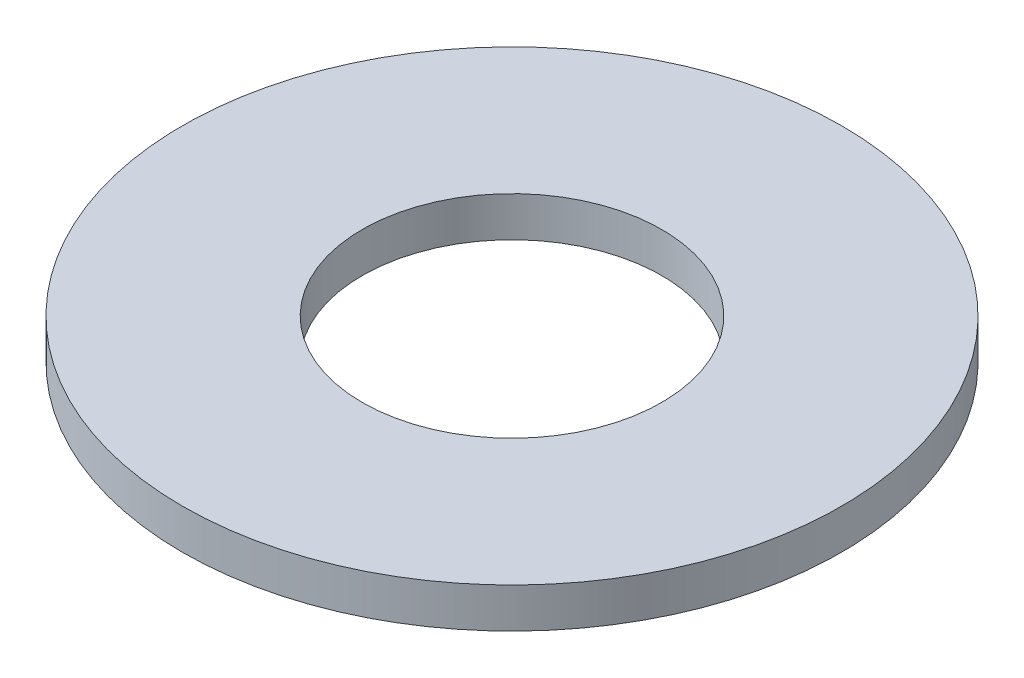
from build123d import *

# Parameters (mm, degrees)
WASHER_PROFILE_165X_75_R   = 82.5
WASHER_PROFILE_165X_75_R_2 = 37.5
WASHER_BODY_10MM_DEPTH     = 10


with BuildPart() as part:
    # Washer Profile Ø165xØ75 → Washer Body 10mm (new body)
    with BuildSketch(Plane(origin=(0, 0, 0), x_dir=(1, 0, 0), z_dir=(0, 1, 0))):
        with Locations(Location((0, 0, 0), (0, 0, 270))):
            Circle(WASHER_PROFILE_165X_75_R)
        with Locations(Location((0, 0, 0), (0, 0, 270))):
            Circle(WASHER_PROFILE_165X_75_R_2, mode=Mode.SUBTRACT)
    extrude(amount=WASHER_BODY_10MM_DEPTH)


solid = part.part
